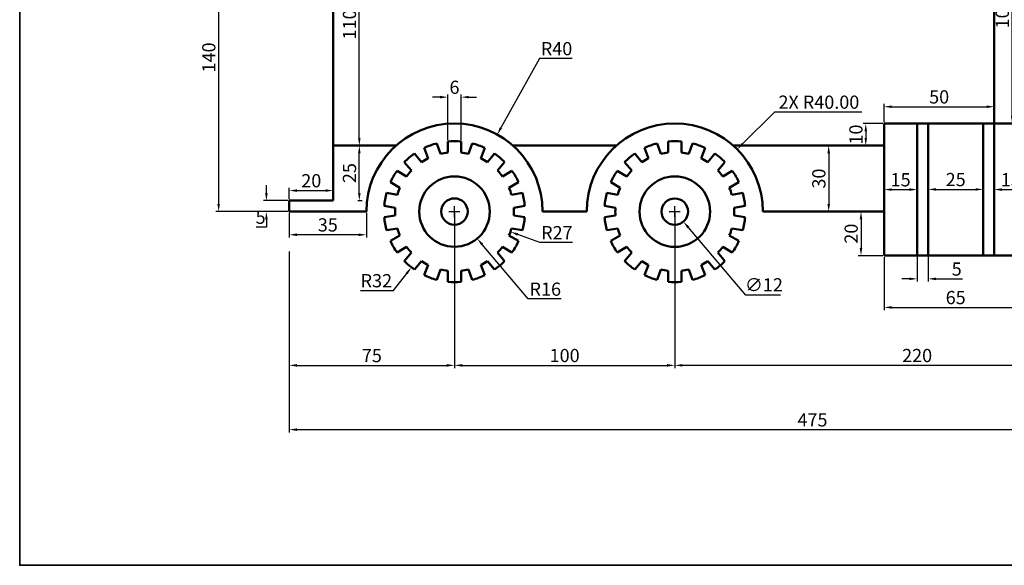
# Model space of a CAD drawing. Units: millimetres. Extents: x -71 to 780, y -41 to 454.
# Tile 1 of 4: x -71 to 376, y -41 to 206. Entities that reach past the tile are written whole.
import ezdxf

# ---------------------------------------------------------------- set-up
doc = ezdxf.new("R2010")
doc.units = ezdxf.units.MM
for name, color, linetype, lineweight in [('M-DIMS', 2, 'Continuous', 25), ('M-OUTL', 7, 'Continuous', 50), ('M-TTLB', 7, 'Continuous', 35)]:
    doc.layers.add(name, color=color, linetype=linetype, lineweight=lineweight)
doc.styles.get("Standard").update_dxf_attribs({"font": 'arial.ttf'})
doc.dimstyles.new('ISO-25', dxfattribs={"dimtxt": 6, "dimasz": 3.5, "dimexe": 1.25, "dimexo": 0.625, "dimtad": 1, "dimtoh": 1, "dimdec": 0, "dimtxsty": 'Standard', "dimcen": 2.5, "dimadec": 0, "dimazin": 0, "dimtfac": 1, "dimtdec": 0, "dimtofl": 0, "dimtmove": 0, "dimatfit": 3, "dimfxl": 1, "dimarcsym": 0})

# ---------------------------------------------------------------- blocks, each defined once
blk = doc.blocks.new('*D1')
at = {"layer": 'Defpoints', "color": 0, "transparency": 16777216}
for p in [(51.38, 101.82), (526.38, 99.32), (526.38, 20.33)]:
    blk.add_point(p, dxfattribs=at)
at = {"layer": 'M-DIMS', "color": 0, "lineweight": -2, "transparency": 16777216}
for p, q in [((51.38, 101.2), (51.38, 19.08)), ((526.38, 98.7), (526.38, 19.08)), ((54.88, 20.33), (522.88, 20.33))]:
    blk.add_line(p, q, dxfattribs=at)
at = {"layer": 'M-DIMS', "color": 0, "transparency": 16777216}
for points in [[(54.88, 20.91), (54.88, 19.74), (51.38, 20.33)], [(522.88, 20.91), (522.88, 19.74), (526.38, 20.33)]]:
    blk.add_solid(points, dxfattribs=at)
at = {"layer": 'M-DIMS', "color": 0, "transparency": 16777216, "insert": (288.88, 24), "char_height": 6, "attachment_point": 5}
blk.add_mtext('475', dxfattribs=at)
blk = doc.blocks.new('*D2')
at = {"layer": 'Defpoints', "color": 0, "transparency": 16777216}
for p in [(126.38, 119.32), (51.38, 60.14), (126.38, 49.52)]:
    blk.add_point(p, dxfattribs=at)
at = {"layer": 'M-DIMS', "color": 0, "lineweight": -2, "transparency": 16777216}
for p, q in [((126.38, 118.7), (126.38, 48.27)), ((51.38, 59.51), (51.38, 48.27)), ((54.88, 49.52), (122.88, 49.52))]:
    blk.add_line(p, q, dxfattribs=at)
at = {"layer": 'M-DIMS', "color": 0, "transparency": 16777216}
for points in [[(54.88, 50.1), (54.88, 48.93), (51.38, 49.52)], [(122.88, 50.1), (122.88, 48.93), (126.38, 49.52)]]:
    blk.add_solid(points, dxfattribs=at)
at = {"layer": 'M-DIMS', "color": 0, "transparency": 16777216, "insert": (88.88, 53.19), "char_height": 6, "attachment_point": 5}
blk.add_mtext('75', dxfattribs=at)
blk = doc.blocks.new('*D3')
at = {"layer": 'Defpoints', "color": 0, "transparency": 16777216}
for p in [(226.38, 119.32), (126.38, 66.43), (226.38, 49.52)]:
    blk.add_point(p, dxfattribs=at)
at = {"layer": 'M-DIMS', "color": 0, "lineweight": -2, "transparency": 16777216}
for p, q in [((226.38, 118.7), (226.38, 48.27)), ((126.38, 65.8), (126.38, 48.27)), ((129.88, 49.52), (222.88, 49.52))]:
    blk.add_line(p, q, dxfattribs=at)
at = {"layer": 'M-DIMS', "color": 0, "transparency": 16777216}
for points in [[(129.88, 50.1), (129.88, 48.93), (126.38, 49.52)], [(222.88, 50.1), (222.88, 48.93), (226.38, 49.52)]]:
    blk.add_solid(points, dxfattribs=at)
at = {"layer": 'M-DIMS', "color": 0, "transparency": 16777216, "insert": (176.38, 53.21), "char_height": 6, "attachment_point": 5}
blk.add_mtext('100', dxfattribs=at)
blk = doc.blocks.new('*D4')
at = {"layer": 'Defpoints', "color": 0, "transparency": 16777216}
for p in [(446.38, 119.32), (226.38, 64.35), (226.38, 49.52)]:
    blk.add_point(p, dxfattribs=at)
at = {"layer": 'M-DIMS', "color": 0, "lineweight": -2, "transparency": 16777216}
for p, q in [((446.38, 118.7), (446.38, 48.27)), ((226.38, 63.72), (226.38, 48.27)), ((442.88, 49.52), (229.88, 49.52))]:
    blk.add_line(p, q, dxfattribs=at)
at = {"layer": 'M-DIMS', "color": 0, "transparency": 16777216}
for points in [[(229.88, 50.1), (229.88, 48.93), (226.38, 49.52)], [(442.88, 50.1), (442.88, 48.93), (446.38, 49.52)]]:
    blk.add_solid(points, dxfattribs=at)
at = {"layer": 'M-DIMS', "color": 0, "transparency": 16777216, "insert": (336.38, 53.21), "char_height": 6, "attachment_point": 5}
blk.add_mtext('220', dxfattribs=at)
blk = doc.blocks.new('*D7')
at = {"layer": 'Defpoints', "color": 0, "transparency": 16777216}
for p in [(51.38, 119.32), (86.38, 119.32), (51.38, 108.81)]:
    blk.add_point(p, dxfattribs=at)
at = {"layer": 'M-DIMS', "color": 0, "lineweight": -2, "transparency": 16777216}
for p, q in [((51.38, 118.7), (51.38, 107.56)), ((86.38, 118.7), (86.38, 107.56)), ((82.88, 108.81), (54.88, 108.81))]:
    blk.add_line(p, q, dxfattribs=at)
at = {"layer": 'M-DIMS', "color": 0, "transparency": 16777216}
for points in [[(54.88, 109.4), (54.88, 108.23), (51.38, 108.81)], [(82.88, 109.4), (82.88, 108.23), (86.38, 108.81)]]:
    blk.add_solid(points, dxfattribs=at)
at = {"layer": 'M-DIMS', "color": 0, "transparency": 16777216, "insert": (68.88, 112.51), "char_height": 6, "attachment_point": 5}
blk.add_mtext('35', dxfattribs=at)
blk = doc.blocks.new('*D8')
at = {"layer": 'Defpoints', "color": 0, "transparency": 16777216}
for p in [(51.38, 124.32), (41, 119.32), (51.38, 119.32)]:
    blk.add_point(p, dxfattribs=at)
at = {"layer": 'M-DIMS', "color": 0, "lineweight": -2, "transparency": 16777216}
for p, q in [((41, 127.82), (41, 131.32)), ((50.76, 124.32), (39.75, 124.32)), ((50.76, 119.32), (39.75, 119.32)), ((41, 112.32), (36.39, 112.32)), ((41, 115.82), (41, 112.32))]:
    blk.add_line(p, q, dxfattribs=at)
at = {"layer": 'M-DIMS', "color": 0, "transparency": 16777216}
for points in [[(40.41, 127.82), (41.58, 127.82), (41, 124.32)], [(40.41, 115.82), (41.58, 115.82), (41, 119.32)]]:
    blk.add_solid(points, dxfattribs=at)
at = {"layer": 'M-DIMS', "color": 0, "transparency": 16777216, "insert": (38.38, 116), "char_height": 6, "attachment_point": 5}
blk.add_mtext('5', dxfattribs=at)
blk = doc.blocks.new('*D9')
at = {"layer": 'Defpoints', "color": 0, "transparency": 16777216}
for p in [(71.38, 128.87), (51.38, 124.32), (71.38, 124.32)]:
    blk.add_point(p, dxfattribs=at)
at = {"layer": 'M-DIMS', "color": 0, "lineweight": -2, "transparency": 16777216}
for p, q in [((51.38, 124.95), (51.38, 130.12)), ((71.38, 124.95), (71.38, 130.12)), ((54.88, 128.87), (67.88, 128.87))]:
    blk.add_line(p, q, dxfattribs=at)
at = {"layer": 'M-DIMS', "color": 0, "transparency": 16777216}
for points in [[(54.88, 129.46), (54.88, 128.29), (51.38, 128.87)], [(67.88, 129.46), (67.88, 128.29), (71.38, 128.87)]]:
    blk.add_solid(points, dxfattribs=at)
at = {"layer": 'M-DIMS', "color": 0, "transparency": 16777216, "insert": (61.38, 132.56), "char_height": 6, "attachment_point": 5}
blk.add_mtext('20', dxfattribs=at)
blk = doc.blocks.new('*D10')
at = {"layer": 'Defpoints', "color": 0, "transparency": 16777216}
for p in [(37.81, 259.32), (19.33, 119.32), (37.81, 119.32)]:
    blk.add_point(p, dxfattribs=at)
at = {"layer": 'M-DIMS', "color": 0, "lineweight": -2, "transparency": 16777216}
for p, q in [((37.19, 259.32), (18.08, 259.32)), ((19.33, 255.82), (19.33, 122.82)), ((37.19, 119.32), (18.08, 119.32))]:
    blk.add_line(p, q, dxfattribs=at)
at = {"layer": 'M-DIMS', "color": 0, "transparency": 16777216}
for points in [[(18.74, 255.82), (19.91, 255.82), (19.33, 259.32)], [(18.74, 122.82), (19.91, 122.82), (19.33, 119.32)]]:
    blk.add_solid(points, dxfattribs=at)
at = {"layer": 'M-DIMS', "color": 0, "transparency": 16777216, "insert": (15.64, 189.32), "char_height": 6, "attachment_point": 5, "rotation": 90}
blk.add_mtext('140', dxfattribs=at)
blk = doc.blocks.new('*D11')
at = {"layer": 'Defpoints', "color": 0, "transparency": 16777216}
for p in [(82.72, 259.32), (83.19, 259.32), (82.72, 149.32)]:
    blk.add_point(p, dxfattribs=at)
at = {"layer": 'M-DIMS', "color": 0, "lineweight": -2, "transparency": 16777216}
for p, q in [((83.35, 259.32), (84.44, 259.32)), ((83.19, 152.82), (83.19, 255.82)), ((83.35, 149.32), (84.44, 149.32))]:
    blk.add_line(p, q, dxfattribs=at)
at = {"layer": 'M-DIMS', "color": 0, "transparency": 16777216}
for points in [[(82.61, 255.82), (83.77, 255.82), (83.19, 259.32)], [(82.61, 152.82), (83.77, 152.82), (83.19, 149.32)]]:
    blk.add_solid(points, dxfattribs=at)
at = {"layer": 'M-DIMS', "color": 0, "transparency": 16777216, "insert": (79.5, 204.32), "char_height": 6, "attachment_point": 5, "rotation": 90}
blk.add_mtext('110', dxfattribs=at)
blk = doc.blocks.new('*D12')
at = {"layer": 'Defpoints', "color": 0, "transparency": 16777216}
for p in [(81.86, 149.32), (83.19, 149.32), (81.86, 124.32)]:
    blk.add_point(p, dxfattribs=at)
at = {"layer": 'M-DIMS', "color": 0, "lineweight": -2, "transparency": 16777216}
for p, q in [((82.48, 149.32), (84.44, 149.32)), ((83.19, 127.82), (83.19, 145.82)), ((82.48, 124.32), (84.44, 124.32))]:
    blk.add_line(p, q, dxfattribs=at)
at = {"layer": 'M-DIMS', "color": 0, "transparency": 16777216}
for points in [[(82.61, 145.82), (83.77, 145.82), (83.19, 149.32)], [(82.61, 127.82), (83.77, 127.82), (83.19, 124.32)]]:
    blk.add_solid(points, dxfattribs=at)
at = {"layer": 'M-DIMS', "color": 0, "transparency": 16777216, "insert": (79.5, 136.82), "char_height": 6, "attachment_point": 5, "rotation": 90}
blk.add_mtext('25', dxfattribs=at)
blk = doc.blocks.new('*D33')
at = {"layer": 'Defpoints', "color": 0, "transparency": 16777216}
for p in [(296.24, 149.32), (296.24, 119.32), (296.24, 119.32)]:
    blk.add_point(p, dxfattribs=at)
at = {"layer": 'M-DIMS', "color": 0, "lineweight": -2, "transparency": 16777216}
for p, q in [((296.87, 149.32), (297.49, 149.32)), ((296.24, 145.82), (296.24, 122.82)), ((296.87, 119.32), (297.49, 119.32))]:
    blk.add_line(p, q, dxfattribs=at)
at = {"layer": 'M-DIMS', "color": 0, "transparency": 16777216}
for points in [[(295.66, 145.82), (296.83, 145.82), (296.24, 149.32)], [(295.66, 122.82), (296.83, 122.82), (296.24, 119.32)]]:
    blk.add_solid(points, dxfattribs=at)
at = {"layer": 'M-DIMS', "color": 0, "transparency": 16777216, "insert": (292.55, 134.32), "char_height": 6, "attachment_point": 5, "rotation": 90}
blk.add_mtext('30', dxfattribs=at)
blk = doc.blocks.new('*D34')
at = {"layer": 'Defpoints', "color": 0, "transparency": 16777216}
for p in [(321.38, 159.32), (313.07, 149.32), (321.38, 149.32)]:
    blk.add_point(p, dxfattribs=at)
at = {"layer": 'M-DIMS', "color": 0, "lineweight": -2, "transparency": 16777216}
for p, q in [((320.76, 159.32), (311.82, 159.32)), ((313.07, 155.82), (313.07, 152.82)), ((320.76, 149.32), (311.82, 149.32))]:
    blk.add_line(p, q, dxfattribs=at)
at = {"layer": 'M-DIMS', "color": 0, "transparency": 16777216}
for points in [[(312.49, 155.82), (313.65, 155.82), (313.07, 159.32)], [(312.49, 152.82), (313.65, 152.82), (313.07, 149.32)]]:
    blk.add_solid(points, dxfattribs=at)
at = {"layer": 'M-DIMS', "color": 0, "transparency": 16777216, "insert": (309.38, 154.32), "char_height": 6, "attachment_point": 5, "rotation": 90}
blk.add_mtext('10', dxfattribs=at)
blk = doc.blocks.new('*D35')
at = {"layer": 'Defpoints', "color": 0, "transparency": 16777216}
for p in [(371.38, 166.95), (321.38, 159.32), (371.38, 159.32)]:
    blk.add_point(p, dxfattribs=at)
at = {"layer": 'M-DIMS', "color": 0, "lineweight": -2, "transparency": 16777216}
for p, q in [((321.38, 159.95), (321.38, 168.2)), ((324.88, 166.95), (367.88, 166.95)), ((371.38, 159.95), (371.38, 168.2))]:
    blk.add_line(p, q, dxfattribs=at)
at = {"layer": 'M-DIMS', "color": 0, "transparency": 16777216}
for points in [[(324.88, 167.53), (324.88, 166.37), (321.38, 166.95)], [(367.88, 167.53), (367.88, 166.37), (371.38, 166.95)]]:
    blk.add_solid(points, dxfattribs=at)
at = {"layer": 'M-DIMS', "color": 0, "transparency": 16777216, "insert": (346.38, 170.64), "char_height": 6, "attachment_point": 5}
blk.add_mtext('50', dxfattribs=at)
blk = doc.blocks.new('*D36')
at = {"layer": 'Defpoints', "color": 0, "transparency": 16777216}
for p in [(321.38, 99.32), (386.38, 99.32), (386.38, 75.83)]:
    blk.add_point(p, dxfattribs=at)
at = {"layer": 'M-DIMS', "color": 0, "lineweight": -2, "transparency": 16777216}
for p, q in [((321.38, 98.7), (321.38, 74.58)), ((386.38, 98.7), (386.38, 74.58)), ((324.88, 75.83), (382.88, 75.83))]:
    blk.add_line(p, q, dxfattribs=at)
at = {"layer": 'M-DIMS', "color": 0, "transparency": 16777216}
for points in [[(324.88, 76.42), (324.88, 75.25), (321.38, 75.83)], [(382.88, 76.42), (382.88, 75.25), (386.38, 75.83)]]:
    blk.add_solid(points, dxfattribs=at)
at = {"layer": 'M-DIMS', "color": 0, "transparency": 16777216, "insert": (353.88, 79.52), "char_height": 6, "attachment_point": 5}
blk.add_mtext('65', dxfattribs=at)
blk = doc.blocks.new('*D37')
at = {"layer": 'Defpoints', "color": 0, "transparency": 16777216}
for p in [(321.38, 129.32), (336.38, 129.32), (336.38, 129.32)]:
    blk.add_point(p, dxfattribs=at)
at = {"layer": 'M-DIMS', "color": 0, "lineweight": -2, "transparency": 16777216}
for p, q in [((321.38, 129.95), (321.38, 130.57)), ((336.38, 129.95), (336.38, 130.57)), ((324.88, 129.32), (332.88, 129.32))]:
    blk.add_line(p, q, dxfattribs=at)
at = {"layer": 'M-DIMS', "color": 0, "transparency": 16777216}
for points in [[(324.88, 129.91), (324.88, 128.74), (321.38, 129.32)], [(332.88, 129.91), (332.88, 128.74), (336.38, 129.32)]]:
    blk.add_solid(points, dxfattribs=at)
at = {"layer": 'M-DIMS', "color": 0, "transparency": 16777216, "insert": (328.88, 133.01), "char_height": 6, "attachment_point": 5}
blk.add_mtext('15', dxfattribs=at)
blk = doc.blocks.new('*D38')
at = {"layer": 'Defpoints', "color": 0, "transparency": 16777216}
for p in [(336.38, 114.51), (341.38, 114.51), (341.38, 88.79)]:
    blk.add_point(p, dxfattribs=at)
at = {"layer": 'M-DIMS', "color": 0, "lineweight": -2, "transparency": 16777216}
for p, q in [((336.38, 113.88), (336.38, 87.54)), ((341.38, 113.88), (341.38, 87.54)), ((332.88, 88.79), (329.38, 88.79)), ((344.88, 88.79), (356.94, 88.79))]:
    blk.add_line(p, q, dxfattribs=at)
at = {"layer": 'M-DIMS', "color": 0, "transparency": 16777216}
for points in [[(332.88, 89.37), (332.88, 88.21), (336.38, 88.79)], [(344.88, 89.37), (344.88, 88.21), (341.38, 88.79)]]:
    blk.add_solid(points, dxfattribs=at)
at = {"layer": 'M-DIMS', "color": 0, "transparency": 16777216, "insert": (354.33, 92.47), "char_height": 6, "attachment_point": 5}
blk.add_mtext('5', dxfattribs=at)
blk = doc.blocks.new('*D39')
at = {"layer": 'Defpoints', "color": 0, "transparency": 16777216}
for p in [(341.38, 147.65), (366.38, 147.65), (366.38, 129.41)]:
    blk.add_point(p, dxfattribs=at)
at = {"layer": 'M-DIMS', "color": 0, "lineweight": -2, "transparency": 16777216}
for p, q in [((341.38, 147.02), (341.38, 128.16)), ((366.38, 147.02), (366.38, 128.16)), ((344.88, 129.41), (362.88, 129.41))]:
    blk.add_line(p, q, dxfattribs=at)
at = {"layer": 'M-DIMS', "color": 0, "transparency": 16777216}
for points in [[(344.88, 129.99), (344.88, 128.82), (341.38, 129.41)], [(362.88, 129.99), (362.88, 128.82), (366.38, 129.41)]]:
    blk.add_solid(points, dxfattribs=at)
at = {"layer": 'M-DIMS', "color": 0, "transparency": 16777216, "insert": (353.88, 133.1), "char_height": 6, "attachment_point": 5}
blk.add_mtext('25', dxfattribs=at)
blk = doc.blocks.new('*D40')
at = {"layer": 'Defpoints', "color": 0, "transparency": 16777216}
for p in [(371.38, 129.32), (386.38, 129.32), (386.38, 129.32)]:
    blk.add_point(p, dxfattribs=at)
at = {"layer": 'M-DIMS', "color": 0, "lineweight": -2, "transparency": 16777216}
for p, q in [((371.38, 129.95), (371.38, 130.57)), ((386.38, 129.95), (386.38, 130.57)), ((374.88, 129.32), (382.88, 129.32))]:
    blk.add_line(p, q, dxfattribs=at)
at = {"layer": 'M-DIMS', "color": 0, "transparency": 16777216}
for points in [[(374.88, 129.91), (374.88, 128.74), (371.38, 129.32)], [(382.88, 129.91), (382.88, 128.74), (386.38, 129.32)]]:
    blk.add_solid(points, dxfattribs=at)
at = {"layer": 'M-DIMS', "color": 0, "transparency": 16777216, "insert": (378.88, 133.01), "char_height": 6, "attachment_point": 5}
blk.add_mtext('15', dxfattribs=at)
blk = doc.blocks.new('*D41')
at = {"layer": 'Defpoints', "color": 0, "transparency": 16777216}
for p in [(321.38, 119.32), (310.91, 99.32), (321.38, 99.32)]:
    blk.add_point(p, dxfattribs=at)
at = {"layer": 'M-DIMS', "color": 0, "lineweight": -2, "transparency": 16777216}
for p, q in [((320.76, 119.32), (309.66, 119.32)), ((310.91, 115.82), (310.91, 102.82)), ((320.76, 99.32), (309.66, 99.32))]:
    blk.add_line(p, q, dxfattribs=at)
at = {"layer": 'M-DIMS', "color": 0, "transparency": 16777216}
for points in [[(310.32, 115.82), (311.49, 115.82), (310.91, 119.32)], [(310.32, 102.82), (311.49, 102.82), (310.91, 99.32)]]:
    blk.add_solid(points, dxfattribs=at)
at = {"layer": 'M-DIMS', "color": 0, "transparency": 16777216, "insert": (307.22, 109.32), "char_height": 6, "attachment_point": 5, "rotation": 90}
blk.add_mtext('20', dxfattribs=at)
blk = doc.blocks.new('*D68')
at = {"layer": 'Defpoints', "color": 0, "transparency": 16777216}
for p in [(145.77, 154.31), (126.38, 119.32)]:
    blk.add_point(p, dxfattribs=at)
at = {"layer": 'M-DIMS', "color": 0, "lineweight": -2, "transparency": 16777216}
for p, q in [((164.91, 188.84), (147.47, 157.37)), ((179.85, 188.84), (164.91, 188.84)), ((126.38, 116.82), (126.38, 121.82)), ((123.88, 119.32), (128.88, 119.32))]:
    blk.add_line(p, q, dxfattribs=at)
at = {"layer": 'M-DIMS', "color": 0, "transparency": 16777216}
blk.add_solid([(146.96, 157.65), (147.98, 157.09), (145.77, 154.31)], dxfattribs=at)
at = {"layer": 'M-DIMS', "color": 0, "transparency": 16777216, "insert": (172.7, 192.53), "char_height": 6, "attachment_point": 5}
blk.add_mtext('R40', dxfattribs=at)
blk = doc.blocks.new('*D69')
at = {"layer": 'Defpoints', "color": 0, "transparency": 16777216}
for p in [(126.38, 119.32), (136.69, 107.09)]:
    blk.add_point(p, dxfattribs=at)
at = {"layer": 'M-DIMS', "color": 0, "lineweight": -2, "transparency": 16777216}
for p, q in [((126.38, 116.82), (126.38, 121.82)), ((123.88, 119.32), (128.88, 119.32)), ((159.81, 79.65), (138.95, 104.41)), ((174.77, 79.65), (159.81, 79.65))]:
    blk.add_line(p, q, dxfattribs=at)
at = {"layer": 'M-DIMS', "color": 0, "transparency": 16777216}
blk.add_solid([(139.39, 104.79), (138.5, 104.03), (136.69, 107.09)], dxfattribs=at)
at = {"layer": 'M-DIMS', "color": 0, "transparency": 16777216, "insert": (167.6, 83.34), "char_height": 6, "attachment_point": 5}
blk.add_mtext('R16', dxfattribs=at)
blk = doc.blocks.new('*D70')
at = {"layer": 'Defpoints', "color": 0, "transparency": 16777216}
for p in [(126.38, 119.32), (106.82, 94)]:
    blk.add_point(p, dxfattribs=at)
at = {"layer": 'M-DIMS', "color": 0, "lineweight": -2, "transparency": 16777216}
for p, q in [((126.38, 116.82), (126.38, 121.82)), ((123.88, 119.32), (128.88, 119.32)), ((98.68, 83.48), (104.68, 91.23)), ((83.78, 83.48), (98.68, 83.48))]:
    blk.add_line(p, q, dxfattribs=at)
at = {"layer": 'M-DIMS', "color": 0, "transparency": 16777216}
blk.add_solid([(104.22, 91.59), (105.14, 90.88), (106.82, 94)], dxfattribs=at)
at = {"layer": 'M-DIMS', "color": 0, "transparency": 16777216, "insert": (90.92, 87.17), "char_height": 6, "attachment_point": 5}
blk.add_mtext('R32', dxfattribs=at)
blk = doc.blocks.new('*D71')
at = {"layer": 'Defpoints', "color": 0, "transparency": 16777216}
for p in [(126.38, 119.32), (151.78, 110.15)]:
    blk.add_point(p, dxfattribs=at)
at = {"layer": 'M-DIMS', "color": 0, "lineweight": -2, "transparency": 16777216}
for p, q in [((126.38, 116.82), (126.38, 121.82)), ((123.88, 119.32), (128.88, 119.32)), ((165.06, 105.35), (155.07, 108.96)), ((180.02, 105.35), (165.06, 105.35))]:
    blk.add_line(p, q, dxfattribs=at)
at = {"layer": 'M-DIMS', "color": 0, "transparency": 16777216}
blk.add_solid([(155.27, 109.51), (154.87, 108.41), (151.78, 110.15)], dxfattribs=at)
at = {"layer": 'M-DIMS', "color": 0, "transparency": 16777216, "insert": (172.85, 108.99), "char_height": 6, "attachment_point": 5}
blk.add_mtext('R27', dxfattribs=at)
blk = doc.blocks.new('*D72')
at = {"layer": 'Defpoints', "color": 0, "transparency": 16777216}
for p in [(222.49, 123.89), (230.28, 114.76)]:
    blk.add_point(p, dxfattribs=at)
at = {"layer": 'M-DIMS', "color": 0, "lineweight": -2, "transparency": 16777216}
for p, q in [((226.38, 116.82), (226.38, 121.82)), ((223.88, 119.32), (228.88, 119.32)), ((258.68, 81.45), (232.55, 112.1)), ((274.36, 81.45), (258.68, 81.45))]:
    blk.add_line(p, q, dxfattribs=at)
at = {"layer": 'M-DIMS', "color": 0, "transparency": 16777216}
blk.add_solid([(232.99, 112.47), (232.1, 111.72), (230.28, 114.76)], dxfattribs=at)
at = {"layer": 'M-DIMS', "color": 0, "transparency": 16777216, "insert": (266.83, 85.31), "char_height": 6, "attachment_point": 5}
blk.add_mtext('∅12', dxfattribs=at)
blk = doc.blocks.new('*D73')
at = {"layer": 'Defpoints', "color": 0, "transparency": 16777216}
for p in [(129.38, 171.3), (123.38, 151.18), (129.38, 151.18)]:
    blk.add_point(p, dxfattribs=at)
at = {"layer": 'M-DIMS', "color": 0, "lineweight": -2, "transparency": 16777216}
for p, q in [((119.88, 171.3), (116.38, 171.3)), ((123.38, 151.81), (123.38, 172.55)), ((129.38, 151.81), (129.38, 172.55)), ((132.88, 171.3), (136.38, 171.3))]:
    blk.add_line(p, q, dxfattribs=at)
at = {"layer": 'M-DIMS', "color": 0, "transparency": 16777216}
for points in [[(119.88, 171.88), (119.88, 170.72), (123.38, 171.3)], [(132.88, 171.88), (132.88, 170.72), (129.38, 171.3)]]:
    blk.add_solid(points, dxfattribs=at)
at = {"layer": 'M-DIMS', "color": 0, "transparency": 16777216, "insert": (126.38, 174.99), "char_height": 6, "attachment_point": 5}
blk.add_mtext('6', dxfattribs=at)
blk = doc.blocks.new('*D75')
at = {"layer": 'Defpoints', "color": 0, "transparency": 16777216}
for p in [(371.38, 259.32), (379.51, 259.32), (371.38, 159.32)]:
    blk.add_point(p, dxfattribs=at)
at = {"layer": 'M-DIMS', "color": 0, "lineweight": -2, "transparency": 16777216}
for p, q in [((372.01, 259.32), (380.76, 259.32)), ((379.51, 162.82), (379.51, 255.82)), ((372.01, 159.32), (380.76, 159.32))]:
    blk.add_line(p, q, dxfattribs=at)
at = {"layer": 'M-DIMS', "color": 0, "transparency": 16777216}
for points in [[(378.92, 255.82), (380.09, 255.82), (379.51, 259.32)], [(378.92, 162.82), (380.09, 162.82), (379.51, 159.32)]]:
    blk.add_solid(points, dxfattribs=at)
at = {"layer": 'M-DIMS', "color": 0, "transparency": 16777216, "insert": (375.82, 209.32), "char_height": 6, "attachment_point": 5, "rotation": 90}
blk.add_mtext('100', dxfattribs=at)
blk = doc.blocks.new('WHEEL-GEAR')
for p, q in [((25.54, 58.24), (23.82, 62.96)), ((28.9, 58.83), (28.9, 63.86)), ((34.9, 58.83), (34.9, 63.86)), ((38.25, 58.24), (39.97, 62.96)), ((16.95, 54.48), (13.72, 58.33)), ((19.9, 56.19), (18.18, 60.91)), ((43.89, 56.19), (45.61, 60.91)), ((46.85, 54.48), (50.08, 58.33)), ((12.35, 50.63), (9.12, 54.48)), ((51.44, 50.63), (54.67, 54.48)), ((10.16, 48.01), (5.81, 50.53)), ((53.63, 48.01), (57.99, 50.53)), ((7.16, 42.82), (2.81, 45.33)), ((56.63, 42.82), (60.99, 45.33)), ((5.99, 39.61), (1.04, 40.49)), ((57.8, 39.61), (62.75, 40.49)), ((4.95, 33.71), (0, 34.58)), ((58.84, 33.71), (63.79, 34.58)), ((4.95, 30.29), (0, 29.42)), ((58.84, 30.29), (63.79, 29.42)), ((5.99, 24.39), (1.04, 23.51)), ((57.8, 24.39), (62.75, 23.51)), ((7.16, 21.18), (2.81, 18.67)), ((56.63, 21.18), (60.99, 18.67)), ((10.16, 15.99), (5.81, 13.47)), ((53.63, 15.99), (57.99, 13.47)), ((12.35, 13.37), (9.12, 9.52)), ((16.95, 9.52), (13.72, 5.67)), ((46.85, 9.52), (50.08, 5.67)), ((51.44, 13.37), (54.67, 9.52)), ((19.9, 7.81), (18.18, 3.09)), ((25.54, 5.76), (23.82, 1.04)), ((28.9, 5.17), (28.9, 0.14)), ((34.9, 5.17), (34.9, 0.14)), ((38.25, 5.76), (39.97, 1.04)), ((43.89, 7.81), (45.61, 3.09))]:
    blk.add_line(p, q)
for radius in [16, 6]:
    blk.add_circle((31.9, 32), radius)
for radius, start, end in [(32, 104.6206, 115.3794), (32, 84.6206, 95.3794), (32, 64.6206, 75.3794), (32, 124.6206, 135.3794), (27, 96.3794, 103.6206), (27, 76.3794, 83.6206), (32, 44.6206, 55.3794), (27, 116.3794, 123.6206), (27, 56.3794, 63.6206), (32, 144.6206, 155.3794), (27, 136.3794, 143.6206), (27, 36.3794, 43.6206), (32, 24.6206, 35.3794), (32, 164.6206, 175.3794), (27, 156.3794, 163.6206), (27, 16.3794, 23.6206), (32, 4.6206, 15.3794), (27, 176.3794, 183.6206), (27, 356.3794, 3.6206), (32, 184.6206, 195.3794), (32, 344.6206, 355.3794), (27, 196.3794, 203.6206), (27, 336.3794, 343.6206), (32, 204.6206, 215.3794), (32, 324.6206, 335.3794), (27, 216.3794, 223.6206), (27, 316.3794, 323.6206), (32, 224.6206, 235.3794), (27, 236.3794, 243.6206), (27, 296.3794, 303.6206), (32, 304.6206, 315.3794), (27, 256.3794, 263.6206), (27, 276.3794, 283.6206), (32, 244.6206, 255.3794), (32, 264.6206, 275.3794), (32, 284.6206, 295.3794)]:
    blk.add_arc((31.9, 32), radius, start, end)
blk = doc.blocks.new('*D85')
at = {"layer": 'Defpoints', "color": 0, "transparency": 16777216}
for p in [(254.69, 147.59), (226.38, 119.32)]:
    blk.add_point(p, dxfattribs=at)
at = {"layer": 'M-DIMS', "color": 0, "lineweight": -2, "transparency": 16777216}
for p, q in [((271.67, 164.55), (257.16, 150.06)), ((311.26, 164.55), (271.67, 164.55)), ((226.38, 116.82), (226.38, 121.82)), ((223.88, 119.32), (228.88, 119.32))]:
    blk.add_line(p, q, dxfattribs=at)
at = {"layer": 'M-DIMS', "color": 0, "transparency": 16777216}
blk.add_solid([(256.75, 150.47), (257.58, 149.65), (254.69, 147.59)], dxfattribs=at)
at = {"layer": 'M-DIMS', "color": 0, "transparency": 16777216, "insert": (291.78, 168.24), "char_height": 6, "attachment_point": 5}
blk.add_mtext('2X R40.00', dxfattribs=at)

msp = doc.modelspace()

# ---------------------------------------------------------------- linework, layer by layer
at = {"layer": 'M-OUTL'}
for p, q in [((71.384, 124.324), (71.384, 259.324)), ((371.384, 259.324), (371.384, 159.324)), ((321.384, 159.324), (321.384, 99.324)), ((321.384, 159.324), (386.384, 159.324)), ((336.384, 159.324), (336.384, 99.324)), ((341.384, 159.324), (341.384, 99.324)), ((366.384, 159.324), (366.384, 99.324)), ((371.384, 159.324), (371.384, 99.324)), ((71.384, 149.324), (99.927, 149.324)), ((152.842, 149.324), (199.927, 149.324)), ((252.842, 149.324), (321.384, 149.324)), ((51.384, 119.324), (51.384, 124.324)), ((51.384, 124.324), (71.384, 124.324)), ((86.384, 119.324), (51.384, 119.324)), ((166.384, 119.324), (186.384, 119.324)), ((266.384, 119.324), (321.384, 119.324)), ((321.384, 99.324), (386.384, 99.324))]:
    msp.add_line(p, q, dxfattribs=at)
for centre in [(126.384, 119.324), (226.384, 119.324)]:
    msp.add_arc(centre, 40, 0, 180, dxfattribs=at)
at = {"layer": 'M-TTLB'}
msp.add_lwpolyline([(779.526, -41.268), (-70.976, -41.268), (-70.976, 454.198), (779.526, 454.198)], close=True, dxfattribs=at)

# ---------------------------------------------------------------- block references
at = {"layer": 'M-OUTL', "rotation": 140.0000000000001}
msp.add_blockref('WHEEL-GEAR', (171.387, 123.335), dxfattribs=at)
at = {"layer": 'M-OUTL'}
msp.add_blockref('WHEEL-GEAR', (194.488, 87.324), dxfattribs=at)

# ---------------------------------------------------------------- dimensions: what is measured, and where the dimension line sits
at = {"layer": 'M-DIMS'}
for base, p1, p2, picture, middle in [((19.328, 119.324), (37.815, 259.324), (37.815, 119.324), '*D10', (15.639, 189.324)), ((83.19, 259.324), (82.724, 149.324), (82.724, 259.324), '*D11', (79.501, 204.324)), ((379.507, 259.324), (371.384, 159.324), (371.384, 259.324), '*D75', (375.819, 209.324)), ((313.072, 149.324), (321.384, 159.324), (321.384, 149.324), '*D34', (309.383, 154.324)), ((83.19, 149.324), (81.855, 124.324), (81.855, 149.324), '*D12', (79.501, 136.824)), ((296.245, 119.324), (296.245, 149.324), (296.245, 119.324), '*D33', (292.554, 134.324)), ((40.995, 119.324), (51.384, 124.324), (51.384, 119.324), '*D8', (38.381, 116)), ((310.908, 99.324), (321.384, 119.324), (321.384, 99.324), '*D41', (307.219, 109.324))]:
    dim = msp.add_linear_dim(base=base, p1=p1, p2=p2, angle=90, dimstyle='ISO-25', override={"dimclrd": 0, "dimclre": 0, "dimclrt": 0}, dxfattribs=at)
    dim.commit()
    dim.dimension.update_dxf_attribs({"geometry": picture, "text_midpoint": middle})
for mpoint, picture, middle in [((145.775, 154.31), '*D68', (172.696, 188.84)), ((106.817, 94.004), '*D70', (90.919, 83.476)), ((136.692, 107.087), '*D69', (167.599, 79.647)), ((151.777, 110.148), '*D71', (172.849, 105.35))]:
    dim = msp.add_radius_dim(center=(126.384, 119.324), mpoint=mpoint, dimstyle='ISO-25', override={"dimclrd": 0, "dimclre": 0, "dimclrt": 0}, dxfattribs=at)
    dim.commit()
    dim.dimension.update_dxf_attribs({"geometry": picture, "text_midpoint": middle, "dimtype": 164})
for base, p1, p2, picture, middle in [((129.384, 171.3), (123.384, 151.183), (129.384, 151.183), '*D73', (126.384, 174.988)), ((371.384, 166.95), (321.384, 159.324), (371.384, 159.324), '*D35', (346.384, 170.639)), ((366.384, 129.407), (341.384, 147.647), (366.384, 147.647), '*D39', (353.884, 133.095)), ((71.384, 128.872), (51.384, 124.324), (71.384, 124.324), '*D9', (61.384, 132.561)), ((336.384, 129.324), (321.384, 129.324), (336.384, 129.324), '*D37', (328.884, 133.012)), ((386.384, 129.324), (371.384, 129.324), (386.384, 129.324), '*D40', (378.884, 133.012)), ((126.384, 49.517), (51.384, 60.138), (126.384, 119.324), '*D2', (88.884, 53.193)), ((51.384, 108.815), (86.384, 119.324), (51.384, 119.324), '*D7', (68.884, 112.505)), ((226.384, 49.517), (126.384, 66.426), (226.384, 119.324), '*D3', (176.384, 53.205)), ((226.384, 49.517), (446.384, 119.324), (226.384, 64.346), '*D4', (336.384, 53.205)), ((526.384, 20.326), (51.384, 101.824), (526.384, 99.324), '*D1', (288.884, 24.002)), ((386.384, 75.832), (321.384, 99.324), (386.384, 99.324), '*D36', (353.884, 79.52))]:
    dim = msp.add_linear_dim(base=base, p1=p1, p2=p2, dimstyle='ISO-25', override={"dimclrd": 0, "dimclre": 0, "dimclrt": 0}, dxfattribs=at)
    dim.commit()
    dim.dimension.update_dxf_attribs({"geometry": picture, "text_midpoint": middle})
dim = msp.add_radius_dim(center=(226.384, 119.324), mpoint=(254.688, 147.588), text='2X <>', dimstyle='ISO-25', override={"dimdec": 2, "dimlfac": 1, "dimrnd": 0, "dimzin": 0, "dimdsep": 46, "dimlunit": 2}, dxfattribs=at)
dim.commit()
dim.dimension.update_dxf_attribs({"geometry": '*D85', "text_midpoint": (291.777, 164.547), "dimtype": 164})
dim = msp.add_diameter_dim_2p(p1=(222.491, 123.89), p2=(230.277, 114.758), dimstyle='ISO-25', override={"dimclrd": 0, "dimclre": 0, "dimclrt": 0}, dxfattribs=at)
dim.commit()
dim.dimension.update_dxf_attribs({"geometry": '*D72', "text_midpoint": (266.833, 81.45), "dimtype": 163})
dim = msp.add_linear_dim(base=(341.384, 88.792), p1=(336.384, 114.509), p2=(341.384, 114.509), dimstyle='ISO-25', override={"dimclrd": 0, "dimclre": 0, "dimclrt": 0}, dxfattribs=at)
dim.commit()
dim.dimension.update_dxf_attribs({"geometry": '*D38', "text_midpoint": (354.33, 88.792), "dimtype": 160})

doc.saveas('drawing.dxf')
